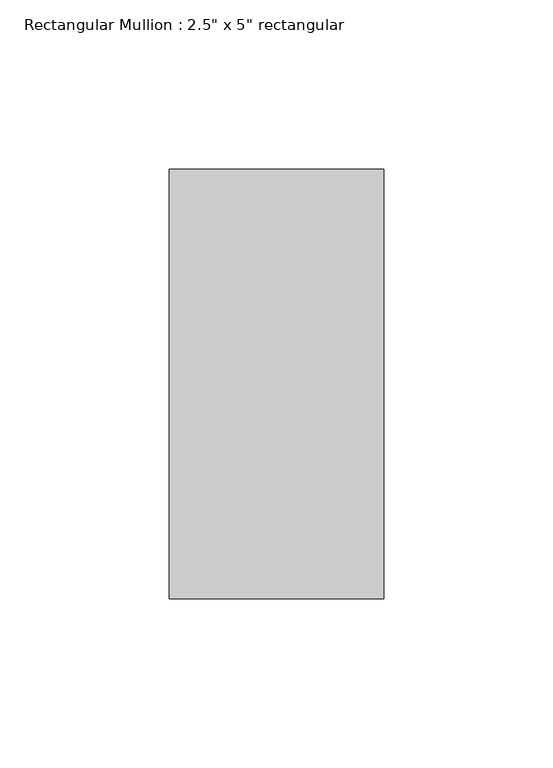
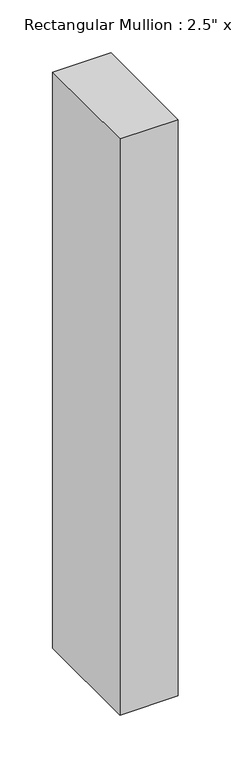
"""IFC4 building model written with IfcOpenShell, lengths in millimetres: member geometry."""

from ifc_helpers import new_model, si_unit, frame, origin, place, context, project, spatial, polyline, outline, extrude, source, transform, mapped, element, save


def member_1a5c3ae3(model_context):
    return source(origin(), model_context, "Body", "SweptSolid", [
        extrude(outline(polyline([(0.0, 63.5), (0.0, -63.5), (-63.5, -63.5), (-63.5, 63.5), (0.0, 63.5)])), frame((0.0, 0.0, -664.6333333), z_axis=(0.0, 0.0, 1.0), x_axis=(1.0, 0.0, 0.0)), (0.0, 0.0, 1.0), 664.6333333),
    ])


if __name__ == "__main__":
    model = new_model("IFC4")
    model_context = context("Model", 3, world=origin())
    ifc_project = project(units=[si_unit("LENGTHUNIT", "METRE", prefix="MILLI")], contexts=[model_context])
    site = spatial("IfcSite", under=ifc_project)
    building = spatial("IfcBuilding", under=site)
    placement = place(None, origin())
    member_shape = member_1a5c3ae3(model_context)
    element("IfcMember", 1, ObjectType="Rectangular Mullion : 2.5\" x 5\" rectangular", at=placement, inside=building, context=model_context, shape_type="MappedRepresentation", body=[
        mapped(member_shape, transform((0.0, 0.0, 0.0), x_axis=(1.0, 0.0, 0.0), y_axis=(0.0, 1.0, 0.0), z_axis=(0.0, 0.0, 1.0))),
    ])
    save(model, "model.ifc")

# Revit data of these elements
# Type "Rectangular Mullion : 2.5\" x 5\" rectangular"
#   built-in parameter 1007304 = 0.416667 (stored number, unit not read)
#   built-in parameter 1007301 = 0.104167 (stored number, unit not read)
#   built-in parameter 1007300 = 0.104167 (stored number, unit not read)
# Element 1 (IfcMember, "Rectangular Mullion : 2.5\" x 5\" rectangular")
#   Materials on its faces: "Aluminum"
# Materials
#   "Aluminum": class "Metal", colour RGB 247 247 247, transparency 0, Description = "Aluminum 6061", Cost = 0
